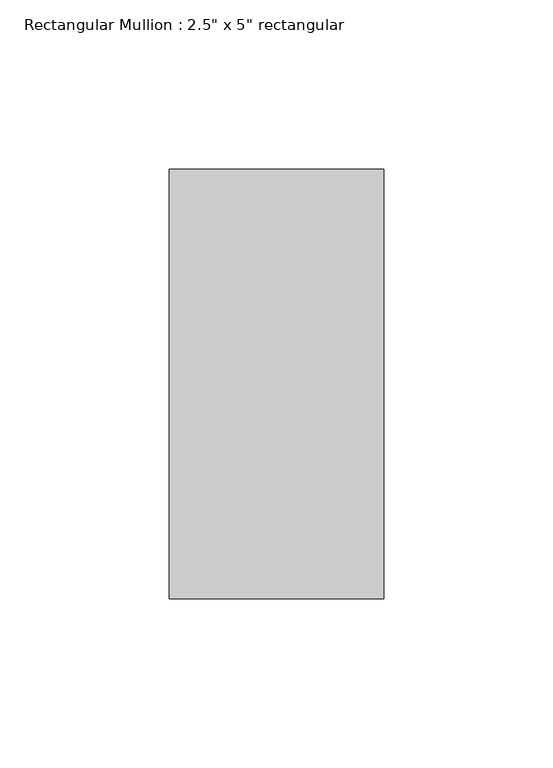
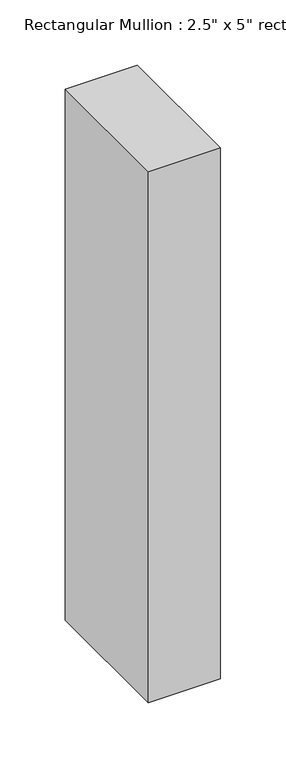
"""IFC4 building model written with IfcOpenShell, lengths in millimetres: member geometry."""

from ifc_helpers import new_model, si_unit, frame, origin, place, context, project, spatial, polyline, outline, extrude, source, transform, mapped, element, save


def member_9ab3e039(model_context):
    return source(origin(), model_context, "Body", "SweptSolid", [
        extrude(outline(polyline([(31.75, 63.5), (31.75, -63.5), (-31.75, -63.5), (-31.75, 63.5), (31.75, 63.5)])), frame((0.0, 0.0, -495.3), z_axis=(0.0, 0.0, 1.0), x_axis=(1.0, 0.0, 0.0)), (0.0, 0.0, 1.0), 495.3),
    ])


if __name__ == "__main__":
    model = new_model("IFC4")
    model_context = context("Model", 3, world=origin())
    ifc_project = project(units=[si_unit("LENGTHUNIT", "METRE", prefix="MILLI")], contexts=[model_context])
    site = spatial("IfcSite", under=ifc_project)
    building = spatial("IfcBuilding", under=site)
    placement = place(None, origin())
    member_shape = member_9ab3e039(model_context)
    element("IfcMember", 1, ObjectType="Rectangular Mullion : 2.5\" x 5\" rectangular", at=placement, inside=building, context=model_context, shape_type="MappedRepresentation", body=[
        mapped(member_shape, transform((0.0, 0.0, 0.0), x_axis=(1.0, 0.0, 0.0), y_axis=(0.0, 1.0, 0.0), z_axis=(0.0, 0.0, 1.0))),
    ])
    save(model, "model.ifc")

# Revit data of these elements
# Type "Rectangular Mullion : 2.5\" x 5\" rectangular"
#   built-in parameter 1007304 = 0.416667 (stored number, unit not read)
#   built-in parameter 1007301 = 0.104167 (stored number, unit not read)
#   built-in parameter 1007300 = 0.104167 (stored number, unit not read)
# Element 1 (IfcMember, "Rectangular Mullion : 2.5\" x 5\" rectangular")
#   Materials on its faces: "Aluminum"
# Materials
#   "Aluminum": class "Metal", colour RGB 247 247 247, transparency 0, Description = "Aluminum 6061", Cost = 0
